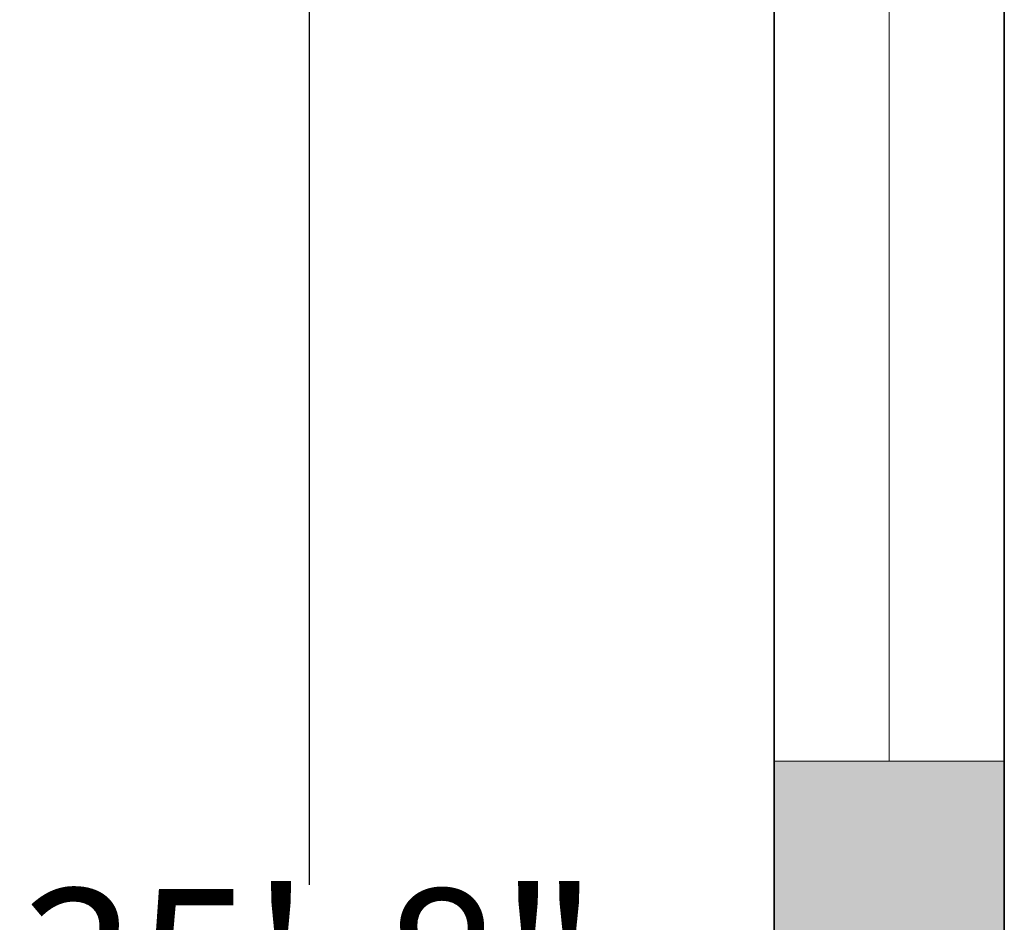
# Model space of a CAD drawing. Units: inches. Extents: x -15 to 423, y -713 to 71.
# Tile 4 of 24: x -4 to 34, y -195 to -159. Entities that reach past the tile are written whole.
import ezdxf

# ---------------------------------------------------------------- set-up
doc = ezdxf.new("R2010")
doc.units = ezdxf.units.IN
doc.header["$MEASUREMENT"] = 0
for name, color, linetype, lineweight in [('A-ANNO-DIMS', 2, 'Continuous', 18), ('A-GLAZ', 5, 'Continuous', 18), ('A-WALL', 7, 'Continuous', 35), ('A-WALL-PATT', 8, 'Continuous', 13)]:
    doc.layers.add(name, color=color, linetype=linetype, lineweight=lineweight)
doc.styles.get("Standard").update_dxf_attribs({"font": 'arial.ttf'})
doc.dimstyles.get("Standard").update_dxf_attribs({"dimtxt": 0.18, "dimasz": 0.18, "dimexe": 0.18, "dimexo": 0.0625, "dimgap": 0.09, "dimtad": 0, "dimtih": 1, "dimtoh": 1, "dimdec": 0, "dimzin": 0, "dimdsep": 46, "dimlunit": 3, "dimtxsty": 'Standard', "dimcen": 0.09, "dimadec": 0, "dimazin": 0, "dimtfac": 1, "dimtdec": 0, "dimtofl": 0, "dimtmove": 0, "dimatfit": 3, "dimfxl": 1, "dimtolj": 1, "dimtzin": 0, "dimarcsym": 0})

# ---------------------------------------------------------------- blocks, each defined once
blk = doc.blocks.new('*D8')
at = {"layer": 'A-ANNO-DIMS', "color": 0, "lineweight": -2, "transparency": 16777216}
for p, q in [((25.018, 17.5), (6.724, 17.5)), ((6.904, 17.32), (6.904, -193.094)), ((6.904, -409.82), (6.904, -199.405)), ((34.018, -410), (6.724, -410))]:
    blk.add_line(p, q, dxfattribs=at)
at = {"layer": 'A-ANNO-DIMS', "color": 0, "transparency": 16777216}
for points in [[(6.874, 17.32), (6.934, 17.32), (6.904, 17.5)], [(6.874, -409.82), (6.934, -409.82), (6.904, -410)]]:
    blk.add_solid(points, dxfattribs=at)
at = {"layer": 'Defpoints', "color": 0, "transparency": 16777216}
for p in [(25.081, 17.5), (6.904, -410), (34.081, -410)]:
    blk.add_point(p, dxfattribs=at)
at = {"layer": 'A-ANNO-DIMS', "color": 0, "transparency": 16777216, "insert": (6.904, -196.25), "char_height": 6, "attachment_point": 5}
blk.add_mtext('\\A1;35\'-8"', dxfattribs=at)
blk = doc.blocks.new('WINDOW-60IN')
for p, q in [((0, 9), (60, 9)), ((0, 0), (0, 9)), ((0, 4.5), (60, 4.5)), ((60, 0), (0, 0))]:
    blk.add_line(p, q)

msp = doc.modelspace()

# ---------------------------------------------------------------- hatches: boundary and pattern name
at = {"layer": 'A-WALL-PATT'}
h = msp.add_hatch(color=256, dxfattribs=at)
h.dxf.hatch_style = 1
h.paths.add_polyline_path([(34.081, -349.58), (25.081, -349.58), (25.081, -431), (34.081, -431)])
h.paths.add_polyline_path([(34.081, -467), (25.081, -467), (25.081, -673), (34.081, -673)])
h.paths.add_polyline_path([(373.081, -668.5), (182.081, -668.5), (182.081, -673), (373.081, -673)])
h.paths.add_polyline_path([(253.199, -597.5), (191.081, -597.5), (191.081, -594.5), (182.081, -594.5), (182.081, -606.5), (253.199, -606.5)])
h.paths.add_polyline_path([(373.081, -597.5), (313.199, -597.5), (313.199, -606.5), (373.081, -606.5)])
h.paths.add_polyline_path([(382.081, -545.549), (373.081, -545.549), (373.081, -673), (382.081, -673)])
h.paths.add_polyline_path([(139.081, -488), (34.081, -488), (34.081, -497), (139.081, -497), (139.081, -492.5)])
h.paths.add_polyline_path([(139.081, -396.5), (128.581, -396.5), (128.581, -352.79), (124.081, -352.79), (124.081, -396.5), (34.081, -396.5), (34.081, -410), (139.081, -410), (139.081, -403.25)])
h.paths.add_polyline_path([(191.081, -396.5), (179.081, -396.5), (179.081, -410), (182.081, -410), (182.081, -488), (179.081, -488), (179.081, -497), (182.081, -497), (182.081, -501.431), (191.081, -501.431)])
h.paths.add_polyline_path([(373.081, -396.5), (253.081, -396.5), (253.081, -393.5), (248.581, -393.5), (248.581, -401), (284.581, -401), (284.581, -404), (289.081, -404), (289.081, -401), (373.081, -401)])
h.paths.add_polyline_path([(373.081, -449), (289.081, -449), (289.081, -432), (286.831, -432), (284.581, -432), (284.581, -453.5), (373.081, -453.5)])
h.paths.add_polyline_path([(382.081, -344.267), (373.081, -344.267), (373.081, -413.683), (382.081, -413.683)])
h.paths.add_polyline_path([(382.081, -437.683), (373.081, -437.683), (373.081, -485.549), (382.081, -485.549)])
h.paths.add_polyline_path([(34.081, -188.264), (25.081, -188.264), (25.081, -289.58), (34.081, -289.58)])
h.paths.add_polyline_path([(164.081, -236), (34.081, -236), (34.081, -240.5), (124.081, -240.5), (124.081, -293.122), (128.581, -293.122), (128.581, -240.5), (164.081, -240.5), (164.081, -238.25)])
h.paths.add_polyline_path([(373.081, -236), (242.581, -236), (242.581, -238.25), (242.581, -240.5), (248.581, -240.5), (248.581, -353.5), (250.831, -353.5), (253.081, -353.5), (253.081, -240.5), (373.081, -240.5)])
h.paths.add_polyline_path([(382.081, -190.86), (373.081, -190.86), (373.081, -284.267), (382.081, -284.267)])
h.paths.add_polyline_path([(211.581, -80), (253.581, -80), (253.581, -77.75), (253.581, -75.5), (153.581, -75.5), (153.581, -77.75), (153.581, -80), (207.081, -80), (207.081, -236), (204.081, -236), (204.081, -240.5), (214.581, -240.5), (214.581, -236), (211.581, -236)])
h.paths.add_polyline_path([(34.081, 8.5), (70.358, 8.5), (70.358, 17.5), (25.081, 17.5), (25.081, -128.264), (34.081, -128.264)])
h.paths.add_polyline_path([(110.581, 17.5), (94.358, 17.5), (94.358, 8.5), (110.581, 8.5)])
h.paths.add_polyline_path([(296.581, 17.5), (110.581, 17.5), (110.581, 13), (296.581, 13)])
h.paths.add_polyline_path([(110.581, 8.5), (106.081, 8.5), (106.081, -75.5), (103.081, -75.5), (103.081, -80), (113.581, -80), (113.581, -77.75), (113.581, -75.5), (110.581, -75.5)])
h.paths.add_polyline_path([(75.081, -75.5), (34.081, -75.5), (34.081, -80), (75.081, -80), (75.081, -77.75)])
h.paths.add_polyline_path([(343.093, 17.5), (296.581, 17.5), (296.581, 13), (296.581, 8.5), (343.093, 8.5)])
h.paths.add_polyline_path([(304.081, -75.5), (301.081, -75.5), (301.081, 8.5), (296.581, 8.5), (296.581, -75.5), (293.581, -75.5), (293.581, -80), (304.081, -80)])
h.paths.add_polyline_path([(382.081, 17.5), (367.093, 17.5), (367.093, 8.5), (373.081, 8.5), (373.081, -130.86), (382.081, -130.86)])
h.paths.add_polyline_path([(373.081, -75.5), (332.081, -75.5), (332.081, -77.75), (332.081, -80), (373.081, -80)])

# ---------------------------------------------------------------- linework, layer by layer
at = {"layer": 'A-WALL'}
for p, q in [((25.081, 17.5), (25.081, -673)), ((34.081, 8.5), (34.081, -673))]:
    msp.add_line(p, q, dxfattribs=at)

# ---------------------------------------------------------------- block references
at = {"layer": 'A-GLAZ', "rotation": 90.00000000000003}
msp.add_blockref('WINDOW-60IN', (34.081, -188.264), dxfattribs=at)

# ---------------------------------------------------------------- dimensions: what is measured, and where the dimension line sits
at = {"layer": 'A-ANNO-DIMS'}
dim = msp.add_linear_dim(base=(6.904132698, -409.999899363), p1=(25.080555734, 17.500100637), p2=(34.080555734, -409.999899363), angle=90, dimstyle='Standard', override={"dimtxt": 6, "dimclrd": 0, "dimclre": 0, "dimclrt": 0}, dxfattribs=at)
dim.commit()
dim.dimension.update_dxf_attribs({"geometry": '*D8', "text_midpoint": (6.904132698, -196.249899363)})

doc.saveas('drawing.dxf')
